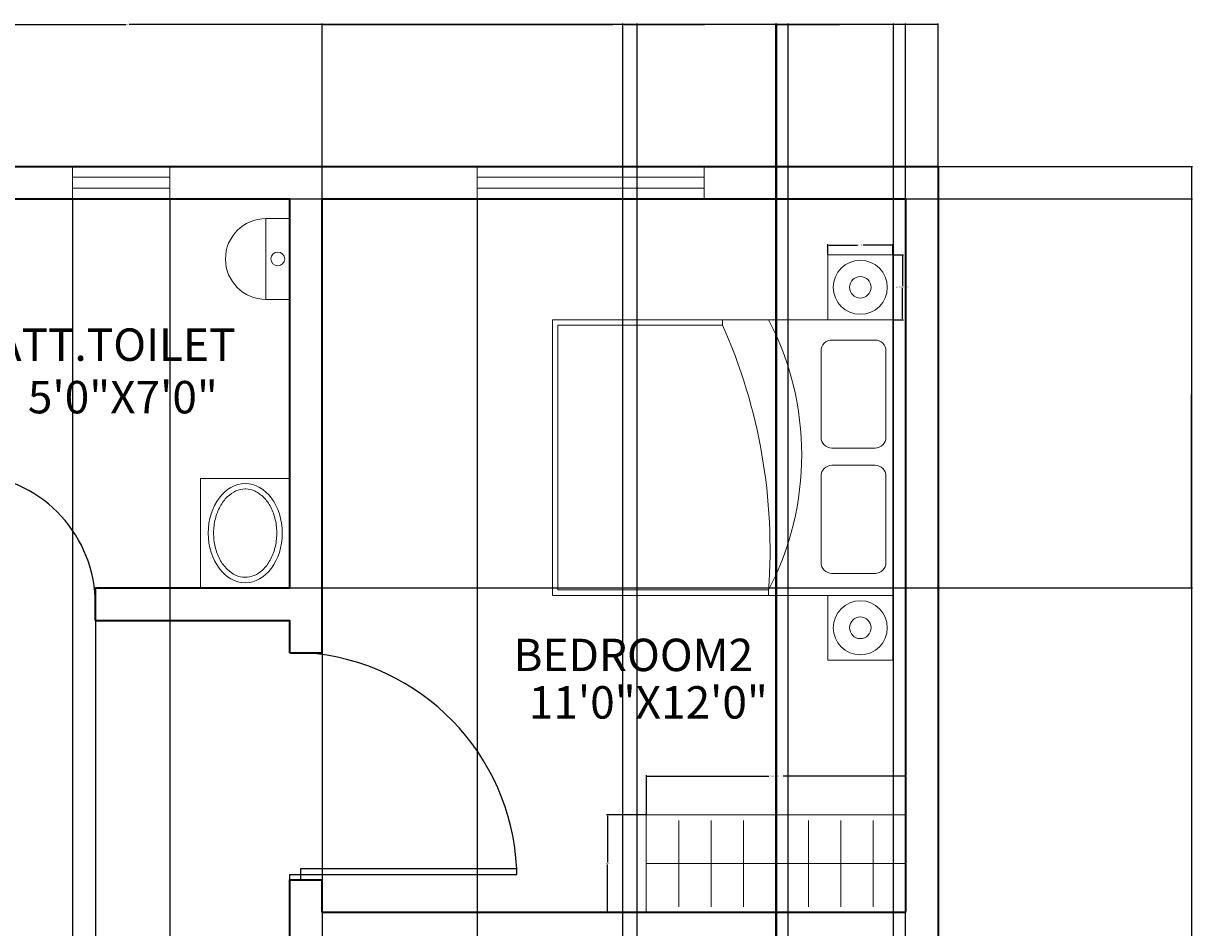
# Model space of a CAD drawing. Units: inches. Extents: x 2608 to 3003, y 1827 to 2396.
# Tile 5 of 5: x 2787 to 3003, y 2229 to 2396. Entities that reach past the tile are written whole.
import ezdxf

# ---------------------------------------------------------------- set-up
doc = ezdxf.new("R2010")
doc.units = ezdxf.units.IN
for name, color, linetype, lineweight in [('A-ANNO-DIMS', 2, 'Continuous', 18), ('A-AREA-IDEN', 7, 'Continuous', 25), ('A-DOOR', 50, 'Continuous', 25), ('A-FLOR-CASE', 213, 'Continuous', 18), ('A-FLOR-FIXT', 213, 'Continuous', 18), ('A-FURN', 254, 'Continuous', 18), ('A-GLAZ', 40, 'Continuous', 18), ('A-WALL', 111, 'Continuous', 35)]:
    doc.layers.add(name, color=color, linetype=linetype, lineweight=lineweight)
doc.styles.get("Standard").update_dxf_attribs({"font": 'arial.ttf'})
doc.dimstyles.get("Standard").update_dxf_attribs({"dimtxt": 0.18, "dimasz": 0.18, "dimexe": 0.18, "dimexo": 0.0625, "dimgap": 0.09, "dimtad": 0, "dimtih": 1, "dimtoh": 1, "dimdec": 4, "dimzin": 0, "dimdsep": 46, "dimtxsty": 'Standard', "dimcen": 0.09, "dimadec": 0, "dimazin": 0, "dimtfac": 1, "dimtdec": 4, "dimtofl": 0, "dimtmove": 0, "dimatfit": 3, "dimfxl": 1, "dimtolj": 1, "dimtzin": 0, "dimarcsym": 0})

# ---------------------------------------------------------------- blocks, each defined once
blk = doc.blocks.new('BED-DOUBLE')
for p, q in [((22.99, 51), (22.99, 50)), ((22.99, 50), (61.99, 50)), ((61.99, 50), (61.99, 1)), ((61.99, 1), (31.5, 1)), ((31.5, 1), (31.5, 0))]:
    blk.add_line(p, q)
blk.add_lwpolyline([(0, 51), (63, 51), (63, 0), (0, 0)], close=True)
for points in [[(3.26, 46.94), (11.26, 46.94, -0.414214), (13.26, 44.94), (13.26, 28.94, -0.414214), (11.26, 26.94), (3.26, 26.94, -0.414214), (1.26, 28.94), (1.26, 44.94, -0.414214)], [(3.26, 23.76), (11.26, 23.76, -0.414214), (13.26, 21.76), (13.26, 5.76, -0.414214), (11.26, 3.76), (3.26, 3.76, -0.414214), (1.26, 5.76), (1.26, 21.76, -0.414214)]]:
    blk.add_lwpolyline(points, format="xyb", close=True)
for centre, radius, start, end in [((70.85, 25), 54, 152.4215, 207.5785), ((124.71, 42.43), 102, 175.743, 203.964)]:
    blk.add_arc(centre, radius, start, end)
blk = doc.blocks.new('NIGHTSTAND-LAMP')
blk.add_lwpolyline([(0, 0), (12, 0), (12, 12), (0, 12)], close=True)
for radius in [5, 2]:
    blk.add_circle((6, 6), radius)
blk = doc.blocks.new('WARDROBE-48')
for p, q in [((48, 18), (0, 18)), ((0, 18), (0, 0)), ((48, 0), (48, 18)), ((6, 1), (6, 17)), ((12, 1), (12, 17)), ((18, 1), (18, 17)), ((24, 1), (24, 17)), ((30, 1), (30, 17)), ((36, 1), (36, 17)), ((42, 1), (42, 17)), ((0, 9), (48, 9)), ((0, 0), (48, 0))]:
    blk.add_line(p, q)
blk = doc.blocks.new('WC-PAN')
blk.add_lwpolyline([(16.51, 0), (0, 0), (0, 20.28), (16.51, 20.28)], close=True)
blk.add_ellipse((8.26, 10.14), major_axis=(0, 9.17), ratio=0.747248)
blk.add_open_spline([(8.26, 18.31), (7.68, 18.31), (7.1, 18.19), (5.98, 17.7), (5.44, 17.34), (4.44, 16.37), (3.98, 15.77), (3.23, 14.38), (2.93, 13.6), (2.52, 11.95), (2.41, 11.07), (2.4, 9.31), (2.5, 8.43), (2.9, 6.77), (3.19, 5.98), (3.94, 4.59), (4.39, 3.98), (5.38, 2.99), (5.92, 2.62), (7.04, 2.11), (7.62, 1.98), (8.77, 1.97), (9.34, 2.08), (10.47, 2.55), (11.02, 2.9), (12.02, 3.85), (12.48, 4.45), (13.25, 5.82), (13.56, 6.59), (13.98, 8.24), (14.09, 9.12), (14.12, 10.88), (14.02, 11.76), (13.64, 13.43), (13.35, 14.22), (12.62, 15.63), (12.18, 16.24), (11.19, 17.24), (10.65, 17.63), (9.53, 18.15), (8.96, 18.29), (8.34, 18.31), (8.3, 18.31), (8.26, 18.31)], degree=3, knots=[0, 0, 0, 0, 0.313014, 0.313014, 0.626027, 0.626027, 0.939041, 0.939041, 1.252055, 1.252055, 1.565069, 1.565069, 1.878082, 1.878082, 2.191096, 2.191096, 2.50411, 2.50411, 2.817124, 2.817124, 3.130137, 3.130137, 3.443151, 3.443151, 3.756165, 3.756165, 4.069179, 4.069179, 4.382192, 4.382192, 4.695206, 4.695206, 5.00822, 5.00822, 5.321234, 5.321234, 5.634247, 5.634247, 5.947261, 5.947261, 6.260275, 6.260275, 6.283185, 6.283185, 6.283185, 6.283185])
blk = doc.blocks.new('BASIN-WALL')
blk.add_lwpolyline([(11.91, 14.94), (7.47, 14.94), (7.47, 0), (11.91, 0)], close=True)
blk.add_circle((9.69, 7.47), 1.27)
blk.add_arc((7.47, 7.47), 7.47, 90, 270)
blk = doc.blocks.new('WIN-42')
for p, q in [((0, 0), (0, 6)), ((42, 0), (42, 6)), ((0, 4), (42, 4)), ((0, 2), (42, 2))]:
    blk.add_line(p, q)
blk = doc.blocks.new('DOOR-LEAF-42')
for p, q in [((0, 1), (0, 2)), ((0, 2), (40, 2)), ((42, 1), (0, 1)), ((40, 2), (40, 0)), ((42, 0), (42, 1))]:
    blk.add_line(p, q)
blk = doc.blocks.new('*D10')
at = {"layer": 'A-ANNO-DIMS', "color": 0, "lineweight": -2, "transparency": 16777216}
for p, q in [((2947.59, 2353.12), (2949.51, 2353.12)), ((2949.33, 2352.94), (2949.33, 2347.3)), ((2949.33, 2341.3), (2949.33, 2346.94)), ((2947.59, 2341.12), (2949.51, 2341.12))]:
    blk.add_line(p, q, dxfattribs=at)
at = {"layer": 'A-ANNO-DIMS', "color": 0, "transparency": 16777216}
for points in [[(2949.3, 2352.94), (2949.36, 2352.94), (2949.33, 2353.12)], [(2949.3, 2341.3), (2949.36, 2341.3), (2949.33, 2341.12)]]:
    blk.add_solid(points, dxfattribs=at)
at = {"layer": 'Defpoints', "color": 0, "transparency": 16777216}
for p in [(2947.53, 2353.12), (2949.33, 2353.12), (2947.53, 2341.12)]:
    blk.add_point(p, dxfattribs=at)
at = {"layer": 'A-ANNO-DIMS', "color": 0, "transparency": 16777216, "insert": (2949.33, 2347.12), "char_height": 0.18, "attachment_point": 5}
blk.add_mtext('\\A1;NIGHTSTAND 12 TYP.', dxfattribs=at)
blk = doc.blocks.new('*D11')
at = {"layer": 'A-ANNO-DIMS', "color": 0, "lineweight": -2, "transparency": 16777216}
for p, q in [((2935.53, 2353.18), (2935.53, 2355.1)), ((2947.53, 2353.18), (2947.53, 2355.1)), ((2935.71, 2354.92), (2941.01, 2354.92)), ((2947.35, 2354.92), (2942.05, 2354.92))]:
    blk.add_line(p, q, dxfattribs=at)
at = {"layer": 'A-ANNO-DIMS', "color": 0, "transparency": 16777216}
for points in [[(2935.71, 2354.95), (2935.71, 2354.89), (2935.53, 2354.92)], [(2947.35, 2354.95), (2947.35, 2354.89), (2947.53, 2354.92)]]:
    blk.add_solid(points, dxfattribs=at)
at = {"layer": 'Defpoints', "color": 0, "transparency": 16777216}
for p in [(2935.53, 2354.92), (2935.53, 2353.12), (2947.53, 2353.12)]:
    blk.add_point(p, dxfattribs=at)
at = {"layer": 'A-ANNO-DIMS', "color": 0, "transparency": 16777216, "insert": (2941.53, 2354.92), "char_height": 0.18, "attachment_point": 5}
blk.add_mtext('\\A1;12 TYP.', dxfattribs=at)
blk = doc.blocks.new('*D16')
at = {"layer": 'A-ANNO-DIMS', "color": 0, "lineweight": -2, "transparency": 16777216}
for p, q in [((2901.92, 2249.55), (2901.92, 2256.87)), ((2902.1, 2256.69), (2924.61, 2256.69)), ((2949.74, 2256.69), (2927.22, 2256.69)), ((2949.92, 2249.55), (2949.92, 2256.87))]:
    blk.add_line(p, q, dxfattribs=at)
at = {"layer": 'A-ANNO-DIMS', "color": 0, "transparency": 16777216}
for points in [[(2902.1, 2256.72), (2902.1, 2256.66), (2901.92, 2256.69)], [(2949.74, 2256.72), (2949.74, 2256.66), (2949.92, 2256.69)]]:
    blk.add_solid(points, dxfattribs=at)
at = {"layer": 'Defpoints', "color": 0, "transparency": 16777216}
for p in [(2901.92, 2256.69), (2901.92, 2249.49), (2949.92, 2249.49)]:
    blk.add_point(p, dxfattribs=at)
at = {"layer": 'A-ANNO-DIMS', "color": 0, "transparency": 16777216, "insert": (2925.92, 2256.69), "char_height": 0.18, "attachment_point": 5}
blk.add_mtext('\\A1;WARDROBE 48 TYP.', dxfattribs=at)
blk = doc.blocks.new('*D17')
at = {"layer": 'A-ANNO-DIMS', "color": 0, "lineweight": -2, "transparency": 16777216}
for p, q in [((2901.85, 2249.49), (2894.54, 2249.49)), ((2894.72, 2249.31), (2894.72, 2240.67)), ((2894.72, 2231.67), (2894.72, 2240.31)), ((2901.85, 2231.49), (2894.54, 2231.49))]:
    blk.add_line(p, q, dxfattribs=at)
at = {"layer": 'A-ANNO-DIMS', "color": 0, "transparency": 16777216}
for points in [[(2894.69, 2249.31), (2894.75, 2249.31), (2894.72, 2249.49)], [(2894.69, 2231.67), (2894.75, 2231.67), (2894.72, 2231.49)]]:
    blk.add_solid(points, dxfattribs=at)
at = {"layer": 'Defpoints', "color": 0, "transparency": 16777216}
for p in [(2901.92, 2249.49), (2894.72, 2231.49), (2901.92, 2231.49)]:
    blk.add_point(p, dxfattribs=at)
at = {"layer": 'A-ANNO-DIMS', "color": 0, "transparency": 16777216, "insert": (2894.72, 2240.49), "char_height": 0.18, "attachment_point": 5}
blk.add_mtext('\\A1;18 TYP.', dxfattribs=at)
blk = doc.blocks.new('*D28')
at = {"layer": 'A-ANNO-DIMS', "color": 0, "lineweight": -2, "transparency": 16777216}
for p, q in [((2655.92, 2191.9), (2655.92, 2395.95)), ((2656.1, 2395.77), (2805.63, 2395.77)), ((2955.74, 2395.77), (2806.2, 2395.77)), ((2955.92, 2201.05), (2955.92, 2395.95))]:
    blk.add_line(p, q, dxfattribs=at)
at = {"layer": 'A-ANNO-DIMS', "color": 0, "transparency": 16777216}
for points in [[(2656.1, 2395.8), (2656.1, 2395.74), (2655.92, 2395.77)], [(2955.74, 2395.8), (2955.74, 2395.74), (2955.92, 2395.77)]]:
    blk.add_solid(points, dxfattribs=at)
at = {"layer": 'Defpoints', "color": 0, "transparency": 16777216}
for p in [(2955.92, 2395.77), (2955.92, 2200.98), (2655.92, 2191.84)]:
    blk.add_point(p, dxfattribs=at)
at = {"layer": 'A-ANNO-DIMS', "color": 0, "transparency": 16777216, "insert": (2805.92, 2395.77), "char_height": 0.18, "attachment_point": 5}
blk.add_mtext('\\A1;300', dxfattribs=at)
blk = doc.blocks.new('*D29')
at = {"layer": 'A-ANNO-DIMS', "color": 0, "lineweight": -2, "transparency": 16777216}
for p, q in [((2955.98, 2369.49), (3003.02, 2369.49)), ((3002.84, 2369.31), (3002.84, 2129.67)), ((3002.84, 1889.67), (3002.84, 2129.31)), ((2955.98, 1889.49), (3003.02, 1889.49))]:
    blk.add_line(p, q, dxfattribs=at)
at = {"layer": 'A-ANNO-DIMS', "color": 0, "transparency": 16777216}
for points in [[(3002.81, 2369.31), (3002.87, 2369.31), (3002.84, 2369.49)], [(3002.81, 1889.67), (3002.87, 1889.67), (3002.84, 1889.49)]]:
    blk.add_solid(points, dxfattribs=at)
at = {"layer": 'Defpoints', "color": 0, "transparency": 16777216}
for p in [(2955.92, 2369.49), (3002.84, 2369.49), (2955.92, 1889.49)]:
    blk.add_point(p, dxfattribs=at)
at = {"layer": 'A-ANNO-DIMS', "color": 0, "transparency": 16777216, "insert": (3002.84, 2129.49), "char_height": 0.18, "attachment_point": 5}
blk.add_mtext('\\A1;480', dxfattribs=at)
blk = doc.blocks.new('*D39')
at = {"layer": 'A-ANNO-DIMS', "color": 0, "lineweight": -2, "transparency": 16777216}
for p, q in [((2841.92, 2363.55), (2841.92, 2395.95)), ((2842.1, 2395.77), (2895.63, 2395.77)), ((2949.74, 2395.77), (2896.2, 2395.77)), ((2949.92, 2363.55), (2949.92, 2395.95))]:
    blk.add_line(p, q, dxfattribs=at)
at = {"layer": 'A-ANNO-DIMS', "color": 0, "transparency": 16777216}
for points in [[(2842.1, 2395.8), (2842.1, 2395.74), (2841.92, 2395.77)], [(2949.74, 2395.8), (2949.74, 2395.74), (2949.92, 2395.77)]]:
    blk.add_solid(points, dxfattribs=at)
at = {"layer": 'Defpoints', "color": 0, "transparency": 16777216}
for p in [(2949.92, 2395.77), (2841.92, 2363.49), (2949.92, 2363.49)]:
    blk.add_point(p, dxfattribs=at)
at = {"layer": 'A-ANNO-DIMS', "color": 0, "transparency": 16777216, "insert": (2895.92, 2395.77), "char_height": 0.18, "attachment_point": 5}
blk.add_mtext('\\A1;108', dxfattribs=at)
blk = doc.blocks.new('*D41')
at = {"layer": 'A-ANNO-DIMS', "color": 0, "lineweight": -2, "transparency": 16777216}
for p, q in [((2835.98, 2363.49), (3003.02, 2363.49)), ((3002.84, 2363.31), (3002.84, 2327.67)), ((3002.84, 2291.67), (3002.84, 2327.31)), ((2835.98, 2291.49), (3003.02, 2291.49))]:
    blk.add_line(p, q, dxfattribs=at)
at = {"layer": 'A-ANNO-DIMS', "color": 0, "transparency": 16777216}
for points in [[(3002.81, 2363.31), (3002.87, 2363.31), (3002.84, 2363.49)], [(3002.81, 2291.67), (3002.87, 2291.67), (3002.84, 2291.49)]]:
    blk.add_solid(points, dxfattribs=at)
at = {"layer": 'Defpoints', "color": 0, "transparency": 16777216}
for p in [(2835.92, 2363.49), (3002.84, 2363.49), (2835.92, 2291.49)]:
    blk.add_point(p, dxfattribs=at)
at = {"layer": 'A-ANNO-DIMS', "color": 0, "transparency": 16777216, "insert": (3002.84, 2327.49), "char_height": 0.18, "attachment_point": 5}
blk.add_mtext('\\A1;72', dxfattribs=at)
blk = doc.blocks.new('*D42')
at = {"layer": 'A-ANNO-DIMS', "color": 0, "lineweight": -2, "transparency": 16777216}
for p, q in [((2775.92, 2285.43), (2775.92, 1827.03)), ((2799.92, 2285.43), (2799.92, 1827.03)), ((2776.1, 1827.21), (2787.7, 1827.21)), ((2799.74, 1827.21), (2788.14, 1827.21))]:
    blk.add_line(p, q, dxfattribs=at)
at = {"layer": 'A-ANNO-DIMS', "color": 0, "transparency": 16777216}
for points in [[(2776.1, 1827.24), (2776.1, 1827.18), (2775.92, 1827.21)], [(2799.74, 1827.24), (2799.74, 1827.18), (2799.92, 1827.21)]]:
    blk.add_solid(points, dxfattribs=at)
at = {"layer": 'Defpoints', "color": 0, "transparency": 16777216}
for p in [(2775.92, 2285.49), (2799.92, 2285.49), (2799.92, 1827.21)]:
    blk.add_point(p, dxfattribs=at)
at = {"layer": 'A-ANNO-DIMS', "color": 0, "transparency": 16777216, "insert": (2787.92, 1827.21), "char_height": 0.18, "attachment_point": 5}
blk.add_mtext('\\A1;24', dxfattribs=at)
blk = doc.blocks.new('*D44')
at = {"layer": 'A-ANNO-DIMS', "color": 0, "lineweight": -2, "transparency": 16777216}
for p, q in [((2775.92, 2363.43), (2775.92, 1827.03)), ((2795.68, 2363.43), (2795.68, 1827.03)), ((2776.1, 1827.21), (2785.34, 1827.21)), ((2795.5, 1827.21), (2786.25, 1827.21))]:
    blk.add_line(p, q, dxfattribs=at)
at = {"layer": 'A-ANNO-DIMS', "color": 0, "transparency": 16777216}
for points in [[(2776.1, 1827.24), (2776.1, 1827.18), (2775.92, 1827.21)], [(2795.5, 1827.24), (2795.5, 1827.18), (2795.68, 1827.21)]]:
    blk.add_solid(points, dxfattribs=at)
at = {"layer": 'Defpoints', "color": 0, "transparency": 16777216}
for p in [(2775.92, 2363.49), (2795.68, 2363.49), (2795.68, 1827.21)]:
    blk.add_point(p, dxfattribs=at)
at = {"layer": 'A-ANNO-DIMS', "color": 0, "transparency": 16777216, "insert": (2785.8, 1827.21), "char_height": 0.18, "attachment_point": 5}
blk.add_mtext('\\A1;19.766', dxfattribs=at)
blk = doc.blocks.new('*D45')
at = {"layer": 'A-ANNO-DIMS', "color": 0, "lineweight": -2, "transparency": 16777216}
for p, q in [((2795.68, 2363.43), (2795.68, 1827.03)), ((2813.68, 2363.43), (2813.68, 1827.03)), ((2795.86, 1827.21), (2804.47, 1827.21)), ((2813.5, 1827.21), (2804.89, 1827.21))]:
    blk.add_line(p, q, dxfattribs=at)
at = {"layer": 'A-ANNO-DIMS', "color": 0, "transparency": 16777216}
for points in [[(2795.86, 1827.24), (2795.86, 1827.18), (2795.68, 1827.21)], [(2813.5, 1827.24), (2813.5, 1827.18), (2813.68, 1827.21)]]:
    blk.add_solid(points, dxfattribs=at)
at = {"layer": 'Defpoints', "color": 0, "transparency": 16777216}
for p in [(2795.68, 2363.49), (2813.68, 2363.49), (2813.68, 1827.21)]:
    blk.add_point(p, dxfattribs=at)
at = {"layer": 'A-ANNO-DIMS', "color": 0, "transparency": 16777216, "insert": (2804.68, 1827.21), "char_height": 0.18, "attachment_point": 5}
blk.add_mtext('\\A1;18', dxfattribs=at)
blk = doc.blocks.new('*D46')
at = {"layer": 'A-ANNO-DIMS', "color": 0, "lineweight": -2, "transparency": 16777216}
for p, q in [((2841.92, 2363.43), (2841.92, 1827.03)), ((2870.61, 2363.43), (2870.61, 1827.03)), ((2842.1, 1827.21), (2855.87, 1827.21)), ((2870.43, 1827.21), (2856.66, 1827.21))]:
    blk.add_line(p, q, dxfattribs=at)
at = {"layer": 'A-ANNO-DIMS', "color": 0, "transparency": 16777216}
for points in [[(2842.1, 1827.24), (2842.1, 1827.18), (2841.92, 1827.21)], [(2870.43, 1827.24), (2870.43, 1827.18), (2870.61, 1827.21)]]:
    blk.add_solid(points, dxfattribs=at)
at = {"layer": 'Defpoints', "color": 0, "transparency": 16777216}
for p in [(2841.92, 2363.49), (2870.61, 2363.49), (2870.61, 1827.21)]:
    blk.add_point(p, dxfattribs=at)
at = {"layer": 'A-ANNO-DIMS', "color": 0, "transparency": 16777216, "insert": (2856.26, 1827.21), "char_height": 0.18, "attachment_point": 5}
blk.add_mtext('\\A1;28.69', dxfattribs=at)
blk = doc.blocks.new('*D54')
at = {"layer": 'A-ANNO-DIMS', "color": 0, "lineweight": -2, "transparency": 16777216}
for p, q in [((2925.92, 2135.55), (2925.92, 2395.95)), ((2926.1, 2395.77), (2937.7, 2395.77)), ((2949.74, 2395.77), (2938.14, 2395.77)), ((2949.92, 2135.55), (2949.92, 2395.95))]:
    blk.add_line(p, q, dxfattribs=at)
at = {"layer": 'A-ANNO-DIMS', "color": 0, "transparency": 16777216}
for points in [[(2926.1, 2395.8), (2926.1, 2395.74), (2925.92, 2395.77)], [(2949.74, 2395.8), (2949.74, 2395.74), (2949.92, 2395.77)]]:
    blk.add_solid(points, dxfattribs=at)
at = {"layer": 'Defpoints', "color": 0, "transparency": 16777216}
for p in [(2949.92, 2395.77), (2925.92, 2135.49), (2949.92, 2135.49)]:
    blk.add_point(p, dxfattribs=at)
at = {"layer": 'A-ANNO-DIMS', "color": 0, "transparency": 16777216, "insert": (2937.92, 2395.77), "char_height": 0.18, "attachment_point": 5}
blk.add_mtext('\\A1;24', dxfattribs=at)
blk = doc.blocks.new('*D57')
at = {"layer": 'A-ANNO-DIMS', "color": 0, "lineweight": -2, "transparency": 16777216}
for p, q in [((2897.55, 2039.55), (2897.55, 2395.95)), ((2897.73, 2395.77), (2911.34, 2395.77)), ((2925.74, 2395.77), (2912.13, 2395.77)), ((2925.92, 2039.55), (2925.92, 2395.95))]:
    blk.add_line(p, q, dxfattribs=at)
at = {"layer": 'A-ANNO-DIMS', "color": 0, "transparency": 16777216}
for points in [[(2897.73, 2395.8), (2897.73, 2395.74), (2897.55, 2395.77)], [(2925.74, 2395.8), (2925.74, 2395.74), (2925.92, 2395.77)]]:
    blk.add_solid(points, dxfattribs=at)
at = {"layer": 'Defpoints', "color": 0, "transparency": 16777216}
for p in [(2925.92, 2395.77), (2897.55, 2039.49), (2925.92, 2039.49)]:
    blk.add_point(p, dxfattribs=at)
at = {"layer": 'A-ANNO-DIMS', "color": 0, "transparency": 16777216, "insert": (2911.73, 2395.77), "char_height": 0.18, "attachment_point": 5}
blk.add_mtext('\\A1;28.37', dxfattribs=at)
blk = doc.blocks.new('*D60')
at = {"layer": 'A-ANNO-DIMS', "color": 0, "lineweight": -2, "transparency": 16777216}
for p, q in [((2928.16, 2110.88), (2928.16, 2395.95)), ((2928.34, 2395.77), (2937.45, 2395.77)), ((2947.47, 2395.77), (2938.36, 2395.77)), ((2947.65, 2110.88), (2947.65, 2395.95))]:
    blk.add_line(p, q, dxfattribs=at)
at = {"layer": 'A-ANNO-DIMS', "color": 0, "transparency": 16777216}
for points in [[(2928.34, 2395.8), (2928.34, 2395.74), (2928.16, 2395.77)], [(2947.47, 2395.8), (2947.47, 2395.74), (2947.65, 2395.77)]]:
    blk.add_solid(points, dxfattribs=at)
at = {"layer": 'Defpoints', "color": 0, "transparency": 16777216}
for p in [(2947.65, 2395.77), (2928.16, 2110.81), (2947.65, 2110.81)]:
    blk.add_point(p, dxfattribs=at)
at = {"layer": 'A-ANNO-DIMS', "color": 0, "transparency": 16777216, "insert": (2937.9, 2395.77), "char_height": 0.18, "attachment_point": 5}
blk.add_mtext('\\A1;19.493', dxfattribs=at)
blk = doc.blocks.new('*D63')
at = {"layer": 'A-ANNO-DIMS', "color": 0, "lineweight": -2, "transparency": 16777216}
for p, q in [((2900.2, 2036.91), (2900.2, 2395.95)), ((2900.38, 2395.77), (2912.67, 2395.77)), ((2925.89, 2395.77), (2913.6, 2395.77)), ((2926.07, 2036.91), (2926.07, 2395.95))]:
    blk.add_line(p, q, dxfattribs=at)
at = {"layer": 'A-ANNO-DIMS', "color": 0, "transparency": 16777216}
for points in [[(2900.38, 2395.8), (2900.38, 2395.74), (2900.2, 2395.77)], [(2925.89, 2395.8), (2925.89, 2395.74), (2926.07, 2395.77)]]:
    blk.add_solid(points, dxfattribs=at)
at = {"layer": 'Defpoints', "color": 0, "transparency": 16777216}
for p in [(2926.07, 2395.77), (2900.2, 2036.85), (2926.07, 2036.85)]:
    blk.add_point(p, dxfattribs=at)
at = {"layer": 'A-ANNO-DIMS', "color": 0, "transparency": 16777216, "insert": (2913.13, 2395.77), "char_height": 0.18, "attachment_point": 5}
blk.add_mtext('\\A1;25.865', dxfattribs=at)

msp = doc.modelspace()

# ---------------------------------------------------------------- linework, layer by layer
at = {"layer": 'A-DOOR'}
for centre, radius, start, end in [((2775.9156, 2288.5438), 24, 359.870639, 85.219955), ((2835.9584, 2237.5938), 42, 2.587052, 85.9625)]:
    msp.add_arc(centre, radius, start, end, dxfattribs=at)
at = {"layer": 'A-GLAZ'}
for p, q in [((2795.6817, 2363.4896), (2795.6817, 2369.4896)), ((2813.6817, 2363.4896), (2813.6817, 2369.4896)), ((2795.6817, 2367.4896), (2813.6817, 2367.4896)), ((2795.6817, 2365.4896), (2813.6817, 2365.4896))]:
    msp.add_line(p, q, dxfattribs=at)
at = {"layer": 'A-WALL'}
for p, q in [((2775.9155, 2363.4896), (2835.9155, 2363.4896)), ((2835.9155, 2291.4896), (2835.9155, 2363.4896)), ((2841.9155, 2279.4896), (2841.9155, 2363.4896)), ((2841.9155, 2363.4896), (2949.9155, 2363.4896)), ((2949.9155, 2363.4896), (2949.9155, 2231.4896)), ((2799.9155, 2291.4896), (2835.9155, 2291.4896)), ((2799.9155, 2285.4896), (2799.9155, 2291.4896)), ((2799.9155, 2285.4896), (2835.9155, 2285.4896)), ((2835.9155, 2279.4896), (2835.9155, 2285.4896)), ((2835.9155, 2279.4896), (2841.9155, 2279.4896)), ((2835.9155, 2225.4896), (2835.9155, 2237.4896)), ((2835.9155, 2237.4896), (2841.9155, 2237.4896)), ((2841.9155, 2231.4896), (2841.9155, 2237.4896)), ((2841.9155, 2231.4896), (2949.9155, 2231.4896))]:
    msp.add_line(p, q, dxfattribs=at)
msp.add_lwpolyline([(2655.9155, 2369.4896), (2955.9155, 2369.4896), (2955.9155, 1889.4896), (2655.9155, 1889.4896)], close=True, dxfattribs=at)

# ---------------------------------------------------------------- block references
at = {"layer": 'A-DOOR', "extrusion": (0, 0, -1), "zscale": -1}
msp.add_blockref('DOOR-LEAF-42', (-2877.9151, 2237.49), dxfattribs=at)
at = {"layer": 'A-FLOR-CASE', "rotation": 180}
msp.add_blockref('WARDROBE-48', (2949.9151, 2249.4892), dxfattribs=at)
at = {"layer": 'A-FLOR-FIXT'}
for name, p in [('BASIN-WALL', (2824.005, 2344.888)), ('WC-PAN', (2819.405, 2291.49))]:
    msp.add_blockref(name, p, dxfattribs=at)
at = {"layer": 'A-FURN'}
for name, p, rotation in [('NIGHTSTAND-LAMP', (2947.5303, 2341.118), 89.99999999998633), ('BED-DOUBLE', (2947.5305, 2341.1181), 180), ('NIGHTSTAND-LAMP', (2947.5305, 2290.1181), 180)]:
    msp.add_blockref(name, p, dxfattribs=dict(at, rotation=rotation))
at = {"layer": 'A-GLAZ'}
msp.add_blockref('WIN-42', (2870.6079, 2363.49), dxfattribs=at)

# ---------------------------------------------------------------- texts
at = {"layer": 'A-AREA-IDEN'}
for tag, p in [('ATT.TOILET', (2781.2685, 2333.5052)), ('5\'0"X7\'0"', (2787.4261, 2323.7921)), ('BEDROOM2', (2877.32, 2276.0968)), ('11\'0"X12\'0"', (2880.1612, 2267.3173))]:
    msp.add_attdef(tag, p, '', height=6, dxfattribs=at)

# ---------------------------------------------------------------- dimensions: what is measured, and where the dimension line sits
at = {"layer": 'A-ANNO-DIMS'}
for base, p1, p2, override, picture, middle in [((2955.9155, 2395.7696), (2655.9155, 2191.8395), (2955.9155, 2200.9836), {"dimdec": 0, "dimlfac": 1, "dimrnd": 0, "dimzin": 0, "dimdsep": 46, "dimlunit": 2}, '*D28', (2805.9155, 2395.7696)), ((2949.9155, 2395.7696), (2841.9155, 2363.4896), (2949.9155, 2363.4896), {"dimdec": 0, "dimlfac": 1, "dimrnd": 0, "dimzin": 0, "dimdsep": 46, "dimlunit": 2}, '*D39', (2895.9155, 2395.7696)), ((2925.9155, 2395.7696), (2897.5458, 2039.4896), (2925.9155, 2039.4896), {"dimdec": 2, "dimlfac": 1, "dimrnd": 0, "dimzin": 0, "dimdsep": 46, "dimlunit": 2}, '*D57', (2911.7307, 2395.7696)), ((2926.0657, 2395.7696), (2900.2006, 2036.8464), (2926.0657, 2036.8464), {"dimdec": 3, "dimlfac": 1, "dimrnd": 0, "dimzin": 0, "dimdsep": 46, "dimlunit": 2}, '*D63', (2913.1332, 2395.7696)), ((2949.9155, 2395.7696), (2925.9155, 2135.4896), (2949.9155, 2135.4896), {"dimdec": 0, "dimlfac": 1, "dimrnd": 0, "dimzin": 0, "dimdsep": 46, "dimlunit": 2}, '*D54', (2937.9155, 2395.7696)), ((2947.6506, 2395.7696), (2928.1576, 2110.8146), (2947.6506, 2110.8146), {"dimdec": 3, "dimlfac": 1, "dimrnd": 0, "dimzin": 0, "dimdsep": 46, "dimlunit": 2}, '*D60', (2937.9041, 2395.7696)), ((2795.6817, 1827.2096), (2775.9155, 2363.4896), (2795.6817, 2363.4896), {"dimdec": 3, "dimlfac": 1, "dimrnd": 0, "dimzin": 0, "dimdsep": 46, "dimlunit": 2}, '*D44', (2785.7986, 1827.2096)), ((2813.6817, 1827.2096), (2795.6817, 2363.4896), (2813.6817, 2363.4896), {"dimdec": 0, "dimlfac": 1, "dimrnd": 0, "dimzin": 0, "dimdsep": 46, "dimlunit": 2}, '*D45', (2804.6817, 1827.2096)), ((2870.6078, 1827.2096), (2841.9155, 2363.4896), (2870.6078, 2363.4896), {"dimdec": 2, "dimlfac": 1, "dimrnd": 0, "dimzin": 0, "dimdsep": 46, "dimlunit": 2}, '*D46', (2856.2616, 1827.2096)), ((2799.9155, 1827.2096), (2775.9155, 2285.4896), (2799.9155, 2285.4896), {"dimdec": 0, "dimlfac": 1, "dimrnd": 0, "dimzin": 0, "dimdsep": 46, "dimlunit": 2}, '*D42', (2787.9155, 1827.2096))]:
    dim = msp.add_linear_dim(base=base, p1=p1, p2=p2, dimstyle='Standard', override=override, dxfattribs=at)
    dim.commit()
    dim.dimension.update_dxf_attribs({"geometry": picture, "text_midpoint": middle})
for base, p1, p2, picture, middle in [((3002.8414, 2369.4896), (2955.9155, 1889.4896), (2955.9155, 2369.4896), '*D29', (3002.8414, 2129.4896)), ((3002.8414, 2363.4896), (2835.9155, 2291.4896), (2835.9155, 2363.4896), '*D41', (3002.8414, 2327.4896))]:
    dim = msp.add_linear_dim(base=base, p1=p1, p2=p2, angle=90, dimstyle='Standard', override={"dimdec": 0, "dimlfac": 1, "dimrnd": 0, "dimzin": 0, "dimdsep": 46, "dimlunit": 2}, dxfattribs=at)
    dim.commit()
    dim.dimension.update_dxf_attribs({"geometry": picture, "text_midpoint": middle})
for base, p1, p2, angle, text, picture, middle in [((2935.5303, 2354.9181), (2947.5303, 2353.1181), (2935.5303, 2353.1181), 180, '<> TYP.', '*D11', (2941.5303, 2354.9181)), ((2949.3303, 2353.1181), (2947.5303, 2341.1181), (2947.5303, 2353.1181), 90, 'NIGHTSTAND <> TYP.', '*D10', (2949.3303, 2347.1181)), ((2901.9155, 2256.6896), (2949.9155, 2249.4896), (2901.9155, 2249.4896), 180, 'WARDROBE <> TYP.', '*D16', (2925.9155, 2256.6896)), ((2894.7155, 2231.4896), (2901.9155, 2249.4896), (2901.9155, 2231.4896), 270, '<> TYP.', '*D17', (2894.7155, 2240.4896))]:
    dim = msp.add_linear_dim(base=base, p1=p1, p2=p2, angle=angle, text=text, dimstyle='Standard', override={"dimdec": 0, "dimlfac": 1, "dimrnd": 0, "dimzin": 0, "dimdsep": 46, "dimlunit": 2}, dxfattribs=at)
    dim.commit()
    dim.dimension.update_dxf_attribs({"geometry": picture, "text_midpoint": middle})

doc.saveas('drawing.dxf')
